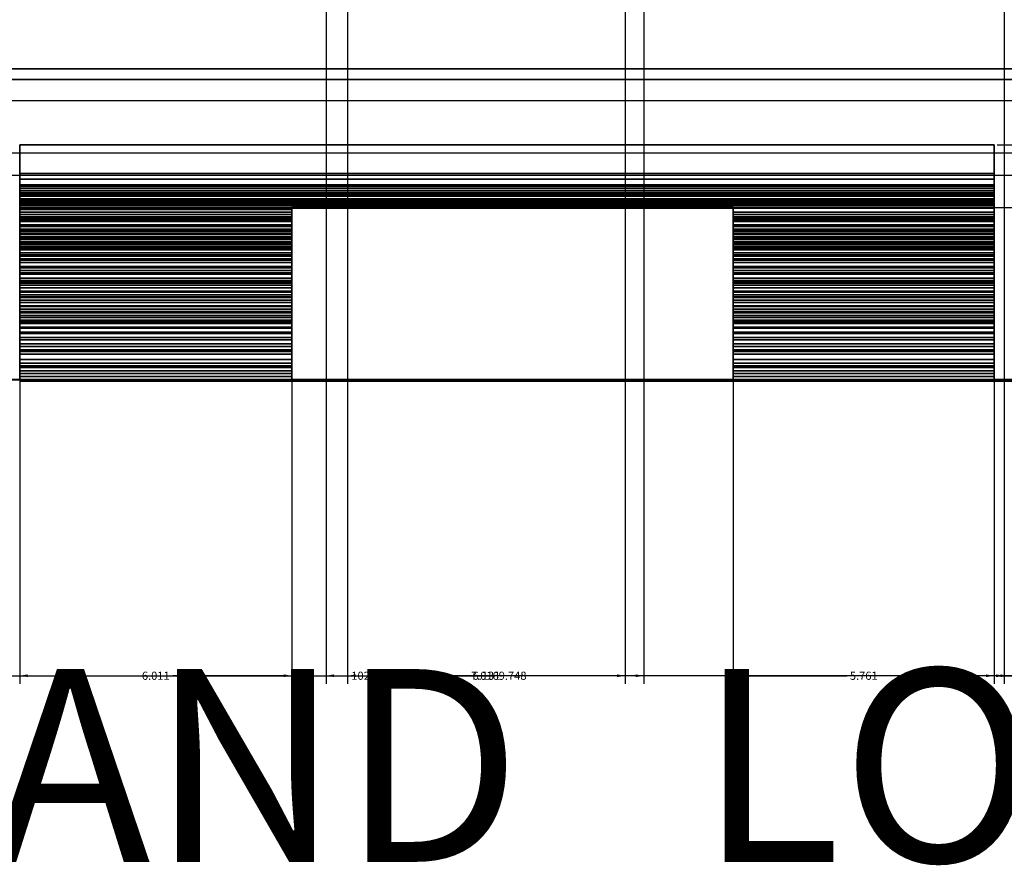
# Model space of a CAD drawing. Units: inches. Extents: x -10 to 130, y -32 to 34.
# Tile 12 of 22: x 49.15 to 70.9, y -32.13 to -13.47. Entities that reach past the tile are written whole.
import ezdxf

# ---------------------------------------------------------------- set-up
doc = ezdxf.new("R2010")
doc.units = ezdxf.units.IN
doc.header["$MEASUREMENT"] = 0
for name, color, linetype, lineweight in [('A-ANNO-DIMS', 2, 'Continuous', 18), ('A-ANNO-TEXT', 7, 'Continuous', 25), ('A-ELEV', 7, 'Continuous', 35)]:
    doc.layers.add(name, color=color, linetype=linetype, lineweight=lineweight)
doc.styles.get("Standard").update_dxf_attribs({"font": 'arial.ttf'})
doc.dimstyles.get("Standard").update_dxf_attribs({"dimtxt": 0.18, "dimasz": 0.18, "dimexe": 0.18, "dimexo": 0.0625, "dimgap": 0.09, "dimtad": 0, "dimtih": 1, "dimtoh": 1, "dimdec": 4, "dimzin": 0, "dimdsep": 46, "dimtxsty": 'Standard', "dimcen": 0.09, "dimadec": 0, "dimazin": 0, "dimtfac": 1, "dimtdec": 4, "dimtofl": 0, "dimtmove": 0, "dimatfit": 3, "dimfxl": 1, "dimtolj": 1, "dimtzin": 0, "dimarcsym": 0})

# ---------------------------------------------------------------- blocks, each defined once
blk = doc.blocks.new('*D1')
at = {"layer": 'A-ANNO-DIMS', "color": 0, "lineweight": -2, "transparency": 16777216}
for p, q in [((5.634, -13.647), (5.634, -28.129)), ((107.933, -21.477), (107.933, -28.129)), ((5.814, -27.949), (56.398, -27.949)), ((107.753, -27.949), (57.169, -27.949))]:
    blk.add_line(p, q, dxfattribs=at)
at = {"layer": 'A-ANNO-DIMS', "color": 0, "transparency": 16777216}
for points in [[(5.814, -27.919), (5.814, -27.979), (5.634, -27.949)], [(107.753, -27.919), (107.753, -27.979), (107.933, -27.949)]]:
    blk.add_solid(points, dxfattribs=at)
at = {"layer": 'Defpoints', "color": 0, "transparency": 16777216}
for p in [(5.634, -13.584), (107.933, -21.414), (107.933, -27.949)]:
    blk.add_point(p, dxfattribs=at)
at = {"layer": 'A-ANNO-DIMS', "color": 0, "transparency": 16777216, "insert": (56.784, -27.949), "char_height": 0.18, "attachment_point": 5}
blk.add_mtext('\\A1;102.3', dxfattribs=at)
blk = doc.blocks.new('*D2')
at = {"layer": 'A-ANNO-DIMS', "color": 0, "lineweight": -2, "transparency": 16777216}
for p, q in [((68.738, 27.199), (129.508, 27.199)), ((129.328, 27.019), (129.328, 3.074)), ((129.328, -21.234), (129.328, 2.71)), ((107.996, -21.414), (129.508, -21.414))]:
    blk.add_line(p, q, dxfattribs=at)
at = {"layer": 'A-ANNO-DIMS', "color": 0, "transparency": 16777216}
for points in [[(129.298, 27.019), (129.358, 27.019), (129.328, 27.199)], [(129.298, -21.234), (129.358, -21.234), (129.328, -21.414)]]:
    blk.add_solid(points, dxfattribs=at)
at = {"layer": 'Defpoints', "color": 0, "transparency": 16777216}
for p in [(68.676, 27.199), (129.328, 27.199), (107.933, -21.414)]:
    blk.add_point(p, dxfattribs=at)
at = {"layer": 'A-ANNO-DIMS', "color": 0, "transparency": 16777216, "insert": (129.328, 2.892), "char_height": 0.18, "attachment_point": 5}
blk.add_mtext('\\A1;48.61', dxfattribs=at)
blk = doc.blocks.new('*D47')
at = {"layer": 'A-ANNO-DIMS', "color": 0, "lineweight": -2, "transparency": 16777216}
for p, q in [((35.567, -12.534), (129.508, -12.534)), ((129.328, -12.714), (129.328, -16.792)), ((129.328, -21.234), (129.328, -17.156)), ((32.034, -21.414), (129.508, -21.414))]:
    blk.add_line(p, q, dxfattribs=at)
at = {"layer": 'A-ANNO-DIMS', "color": 0, "transparency": 16777216}
for points in [[(129.298, -12.714), (129.358, -12.714), (129.328, -12.534)], [(129.298, -21.234), (129.358, -21.234), (129.328, -21.414)]]:
    blk.add_solid(points, dxfattribs=at)
at = {"layer": 'Defpoints', "color": 0, "transparency": 16777216}
for p in [(35.505, -12.534), (31.971, -21.414), (129.328, -21.414)]:
    blk.add_point(p, dxfattribs=at)
at = {"layer": 'A-ANNO-DIMS', "color": 0, "transparency": 16777216, "insert": (129.328, -16.974), "char_height": 0.18, "attachment_point": 5}
blk.add_mtext('\\A1;8.88', dxfattribs=at)
blk = doc.blocks.new('*D52')
at = {"layer": 'A-ANNO-DIMS', "color": 0, "lineweight": -2, "transparency": 16777216}
for p, q in [((49.153, -16.297), (49.153, -28.129)), ((55.165, -17.677), (55.165, -28.129)), ((49.333, -27.949), (51.782, -27.949)), ((54.985, -27.949), (52.536, -27.949))]:
    blk.add_line(p, q, dxfattribs=at)
at = {"layer": 'A-ANNO-DIMS', "color": 0, "transparency": 16777216}
for points in [[(49.333, -27.919), (49.333, -27.979), (49.153, -27.949)], [(54.985, -27.919), (54.985, -27.979), (55.165, -27.949)]]:
    blk.add_solid(points, dxfattribs=at)
at = {"layer": 'Defpoints', "color": 0, "transparency": 16777216}
for p in [(49.153, -16.234), (55.165, -17.615), (55.165, -27.949)]:
    blk.add_point(p, dxfattribs=at)
at = {"layer": 'A-ANNO-DIMS', "color": 0, "transparency": 16777216, "insert": (52.159, -27.949), "char_height": 0.18, "attachment_point": 5}
blk.add_mtext('\\A1;6.011', dxfattribs=at)
blk = doc.blocks.new('*D53')
at = {"layer": 'A-ANNO-DIMS', "color": 0, "lineweight": -2, "transparency": 16777216}
for p, q in [((55.165, -17.677), (55.165, -28.129)), ((64.913, -17.677), (64.913, -28.129)), ((55.345, -27.949), (59.645, -27.949)), ((64.733, -27.949), (60.433, -27.949))]:
    blk.add_line(p, q, dxfattribs=at)
at = {"layer": 'A-ANNO-DIMS', "color": 0, "transparency": 16777216}
for points in [[(55.345, -27.919), (55.345, -27.979), (55.165, -27.949)], [(64.733, -27.919), (64.733, -27.979), (64.913, -27.949)]]:
    blk.add_solid(points, dxfattribs=at)
at = {"layer": 'Defpoints', "color": 0, "transparency": 16777216}
for p in [(55.165, -17.615), (64.913, -17.615), (64.913, -27.949)]:
    blk.add_point(p, dxfattribs=at)
at = {"layer": 'A-ANNO-DIMS', "color": 0, "transparency": 16777216, "insert": (60.039, -27.949), "char_height": 0.18, "attachment_point": 5}
blk.add_mtext('\\A1;9.748', dxfattribs=at)
blk = doc.blocks.new('*D54')
at = {"layer": 'A-ANNO-DIMS', "color": 0, "lineweight": -2, "transparency": 16777216}
for p, q in [((70.674, -16.297), (70.674, -28.129)), ((64.913, -17.677), (64.913, -28.129)), ((65.093, -27.949), (67.417, -27.949)), ((70.494, -27.949), (68.17, -27.949))]:
    blk.add_line(p, q, dxfattribs=at)
at = {"layer": 'A-ANNO-DIMS', "color": 0, "transparency": 16777216}
for points in [[(65.093, -27.919), (65.093, -27.979), (64.913, -27.949)], [(70.494, -27.919), (70.494, -27.979), (70.674, -27.949)]]:
    blk.add_solid(points, dxfattribs=at)
at = {"layer": 'Defpoints', "color": 0, "transparency": 16777216}
for p in [(70.674, -16.234), (64.913, -17.615), (70.674, -27.949)]:
    blk.add_point(p, dxfattribs=at)
at = {"layer": 'A-ANNO-DIMS', "color": 0, "transparency": 16777216, "insert": (67.794, -27.949), "char_height": 0.18, "attachment_point": 5}
blk.add_mtext('\\A1;5.761', dxfattribs=at)
blk = doc.blocks.new('*D55')
at = {"layer": 'A-ANNO-DIMS', "color": 0, "lineweight": -2, "transparency": 16777216}
for p, q in [((72.406, -14.617), (72.406, -28.129)), ((70.674, -16.297), (70.674, -28.129)), ((70.854, -27.949), (71.156, -27.949)), ((72.226, -27.949), (71.925, -27.949))]:
    blk.add_line(p, q, dxfattribs=at)
at = {"layer": 'A-ANNO-DIMS', "color": 0, "transparency": 16777216}
for points in [[(70.854, -27.919), (70.854, -27.979), (70.674, -27.949)], [(72.226, -27.919), (72.226, -27.979), (72.406, -27.949)]]:
    blk.add_solid(points, dxfattribs=at)
at = {"layer": 'Defpoints', "color": 0, "transparency": 16777216}
for p in [(72.406, -14.555), (70.674, -16.234), (72.406, -27.949)]:
    blk.add_point(p, dxfattribs=at)
at = {"layer": 'A-ANNO-DIMS', "color": 0, "transparency": 16777216, "insert": (71.54, -27.949), "char_height": 0.18, "attachment_point": 5}
blk.add_mtext('\\A1;1.732', dxfattribs=at)
blk = doc.blocks.new('*D58')
at = {"layer": 'A-ANNO-DIMS', "color": 0, "lineweight": -2, "transparency": 16777216}
for p, q in [((70.737, -16.234), (129.508, -16.234)), ((129.328, -16.414), (129.328, -18.66)), ((129.328, -21.269), (129.328, -19.024)), ((70.737, -21.449), (129.508, -21.449))]:
    blk.add_line(p, q, dxfattribs=at)
at = {"layer": 'A-ANNO-DIMS', "color": 0, "transparency": 16777216}
for points in [[(129.298, -16.414), (129.358, -16.414), (129.328, -16.234)], [(129.298, -21.269), (129.358, -21.269), (129.328, -21.449)]]:
    blk.add_solid(points, dxfattribs=at)
at = {"layer": 'Defpoints', "color": 0, "transparency": 16777216}
for p in [(70.674, -16.234), (70.674, -21.449), (129.328, -21.449)]:
    blk.add_point(p, dxfattribs=at)
at = {"layer": 'A-ANNO-DIMS', "color": 0, "transparency": 16777216, "insert": (129.328, -18.842), "char_height": 0.18, "attachment_point": 5}
blk.add_mtext('\\A1;5.215', dxfattribs=at)
blk = doc.blocks.new('*D59')
at = {"layer": 'A-ANNO-DIMS', "color": 0, "lineweight": -2, "transparency": 16777216}
for p, q in [((64.975, -17.615), (129.508, -17.615)), ((129.328, -17.795), (129.328, -19.35)), ((129.328, -21.269), (129.328, -19.714)), ((64.975, -21.449), (129.508, -21.449))]:
    blk.add_line(p, q, dxfattribs=at)
at = {"layer": 'A-ANNO-DIMS', "color": 0, "transparency": 16777216}
for points in [[(129.298, -17.795), (129.358, -17.795), (129.328, -17.615)], [(129.298, -21.269), (129.358, -21.269), (129.328, -21.449)]]:
    blk.add_solid(points, dxfattribs=at)
at = {"layer": 'Defpoints', "color": 0, "transparency": 16777216}
for p in [(64.913, -17.615), (64.913, -21.449), (129.328, -21.449)]:
    blk.add_point(p, dxfattribs=at)
at = {"layer": 'A-ANNO-DIMS', "color": 0, "transparency": 16777216, "insert": (129.328, -19.532), "char_height": 0.18, "attachment_point": 5}
blk.add_mtext('\\A1;3.835', dxfattribs=at)
blk = doc.blocks.new('*D64')
at = {"layer": 'A-ANNO-DIMS', "color": 0, "lineweight": -2, "transparency": 16777216}
for p, q in [((82.315, -15.264), (-9.564, -15.264)), ((-9.384, -15.444), (-9.384, -15.659)), ((-9.384, -16.237), (-9.384, -16.022)), ((82.315, -16.417), (-9.564, -16.417))]:
    blk.add_line(p, q, dxfattribs=at)
at = {"layer": 'A-ANNO-DIMS', "color": 0, "transparency": 16777216}
for points in [[(-9.414, -15.444), (-9.354, -15.444), (-9.384, -15.264)], [(-9.414, -16.237), (-9.354, -16.237), (-9.384, -16.417)]]:
    blk.add_solid(points, dxfattribs=at)
at = {"layer": 'Defpoints', "color": 0, "transparency": 16777216}
for p in [(82.377, -15.264), (-9.384, -16.417), (82.377, -16.417)]:
    blk.add_point(p, dxfattribs=at)
at = {"layer": 'A-ANNO-DIMS', "color": 0, "transparency": 16777216, "insert": (-9.384, -15.841), "char_height": 0.18, "attachment_point": 5}
blk.add_mtext('\\A1;1.15', dxfattribs=at)
blk = doc.blocks.new('*D65')
at = {"layer": 'A-ANNO-DIMS', "color": 0, "lineweight": -2, "transparency": 16777216}
for p, q in [((82.315, -16.417), (-9.564, -16.417)), ((-9.384, -16.597), (-9.384, -18.734)), ((-9.384, -21.234), (-9.384, -19.097)), ((80.669, -21.414), (-9.564, -21.414))]:
    blk.add_line(p, q, dxfattribs=at)
at = {"layer": 'A-ANNO-DIMS', "color": 0, "transparency": 16777216}
for points in [[(-9.414, -16.597), (-9.354, -16.597), (-9.384, -16.417)], [(-9.414, -21.234), (-9.354, -21.234), (-9.384, -21.414)]]:
    blk.add_solid(points, dxfattribs=at)
at = {"layer": 'Defpoints', "color": 0, "transparency": 16777216}
for p in [(-9.384, -16.417), (82.377, -16.417), (80.731, -21.414)]:
    blk.add_point(p, dxfattribs=at)
at = {"layer": 'A-ANNO-DIMS', "color": 0, "transparency": 16777216, "insert": (-9.384, -18.916), "char_height": 0.18, "attachment_point": 5}
blk.add_mtext('\\A1;4.998', dxfattribs=at)
blk = doc.blocks.new('*D69')
at = {"layer": 'A-ANNO-DIMS', "color": 0, "lineweight": -2, "transparency": 16777216}
for p, q in [((89.095, -16.906), (-9.564, -16.906)), ((-9.384, -17.086), (-9.384, -18.979)), ((-9.384, -21.234), (-9.384, -19.342)), ((89.095, -21.414), (-9.564, -21.414))]:
    blk.add_line(p, q, dxfattribs=at)
at = {"layer": 'A-ANNO-DIMS', "color": 0, "transparency": 16777216}
for points in [[(-9.414, -17.086), (-9.354, -17.086), (-9.384, -16.906)], [(-9.414, -21.234), (-9.354, -21.234), (-9.384, -21.414)]]:
    blk.add_solid(points, dxfattribs=at)
at = {"layer": 'Defpoints', "color": 0, "transparency": 16777216}
for p in [(89.158, -16.906), (-9.384, -21.414), (89.158, -21.414)]:
    blk.add_point(p, dxfattribs=at)
at = {"layer": 'A-ANNO-DIMS', "color": 0, "transparency": 16777216, "insert": (-9.384, -19.16), "char_height": 0.18, "attachment_point": 5}
blk.add_mtext('\\A1;4.508', dxfattribs=at)
blk = doc.blocks.new('*D72')
at = {"layer": 'A-ANNO-DIMS', "color": 0, "lineweight": -2, "transparency": 16777216}
for p, q in [((55.918, 16.529), (55.918, -28.129)), ((62.934, 16.482), (62.934, -28.129)), ((56.098, -27.949), (59.033, -27.949)), ((62.754, -27.949), (59.819, -27.949))]:
    blk.add_line(p, q, dxfattribs=at)
at = {"layer": 'A-ANNO-DIMS', "color": 0, "transparency": 16777216}
for points in [[(56.098, -27.919), (56.098, -27.979), (55.918, -27.949)], [(62.754, -27.919), (62.754, -27.979), (62.934, -27.949)]]:
    blk.add_solid(points, dxfattribs=at)
at = {"layer": 'Defpoints', "color": 0, "transparency": 16777216}
for p in [(55.918, 16.591), (62.934, 16.545), (62.934, -27.949)]:
    blk.add_point(p, dxfattribs=at)
at = {"layer": 'A-ANNO-DIMS', "color": 0, "transparency": 16777216, "insert": (59.426, -27.949), "char_height": 0.18, "attachment_point": 5}
blk.add_mtext('\\A1;7.016', dxfattribs=at)
blk = doc.blocks.new('*D73')
at = {"layer": 'A-ANNO-DIMS', "color": 0, "lineweight": -2, "transparency": 16777216}
for p, q in [((56.395, 16.255), (56.395, -28.129)), ((62.526, 16.255), (62.526, -28.129)), ((56.575, -27.949), (59.083, -27.949)), ((62.346, -27.949), (59.837, -27.949))]:
    blk.add_line(p, q, dxfattribs=at)
at = {"layer": 'A-ANNO-DIMS', "color": 0, "transparency": 16777216}
for points in [[(56.575, -27.919), (56.575, -27.979), (56.395, -27.949)], [(62.346, -27.919), (62.346, -27.979), (62.526, -27.949)]]:
    blk.add_solid(points, dxfattribs=at)
at = {"layer": 'Defpoints', "color": 0, "transparency": 16777216}
for p in [(56.395, 16.317), (62.526, 16.317), (62.526, -27.949)]:
    blk.add_point(p, dxfattribs=at)
at = {"layer": 'A-ANNO-DIMS', "color": 0, "transparency": 16777216, "insert": (59.46, -27.949), "char_height": 0.18, "attachment_point": 5}
blk.add_mtext('\\A1;6.131', dxfattribs=at)
blk = doc.blocks.new('*D155')
at = {"layer": 'A-ANNO-DIMS', "color": 0, "lineweight": -2, "transparency": 16777216}
for p, q in [((70.897993, 1.448166), (70.897993, -28.129305)), ((71.936707, 1.448166), (71.936707, -28.129305)), ((70.717993, -27.949305), (70.537993, -27.949305)), ((72.116707, -27.949305), (72.296707, -27.949305))]:
    blk.add_line(p, q, dxfattribs=at)
at = {"layer": 'A-ANNO-DIMS', "color": 0, "transparency": 16777216}
for points in [[(70.717993, -27.919305), (70.717993, -27.979305), (70.897993, -27.949305)], [(72.116707, -27.919305), (72.116707, -27.979305), (71.936707, -27.949305)]]:
    blk.add_solid(points, dxfattribs=at)
at = {"layer": 'Defpoints', "color": 0, "transparency": 16777216}
for p in [(70.897993, 1.510666), (71.936707, 1.510666), (71.936707, -27.949305)]:
    blk.add_point(p, dxfattribs=at)
at = {"layer": 'A-ANNO-DIMS', "color": 0, "transparency": 16777216, "insert": (71.41735, -27.949305), "char_height": 0.18, "attachment_point": 5}
blk.add_mtext('\\A1;1.039', dxfattribs=at)

msp = doc.modelspace()

# ---------------------------------------------------------------- linework, layer by layer
at = {"layer": 'A-ELEV'}
for p, q in [((54.1471, -14.555), (47.3492, -14.555)), ((54.1471, -14.555), (64.8443, -14.555)), ((64.8443, -14.555), (72.4063, -14.555)), ((54.1471, -14.7925), (47.3492, -14.7925)), ((54.1471, -14.7925), (64.8443, -14.7925)), ((64.8443, -14.7925), (72.4063, -14.7925)), ((49.1533, -16.2341), (70.6743, -16.2341)), ((49.1533, -16.2341), (49.1533, -21.4145)), ((70.6743, -16.2341), (70.6743, -21.4145)), ((49.1533, -16.867), (70.6743, -16.867)), ((49.1533, -16.987), (70.6743, -16.987)), ((49.1533, -17.1115), (70.6743, -17.1115)), ((49.1533, -17.1249), (70.6743, -17.1249)), ((49.1533, -17.1447), (70.6743, -17.1447)), ((49.1533, -17.1843), (70.6743, -17.1843)), ((49.1533, -17.236), (70.6743, -17.236)), ((49.1533, -17.2835), (70.6743, -17.2835)), ((49.1533, -17.3231), (70.6743, -17.3231)), ((49.1533, -17.3427), (70.6743, -17.3427)), ((49.1533, -17.3429), (70.6743, -17.3429)), ((49.1533, -17.3628), (70.6743, -17.3628)), ((49.1533, -17.4222), (70.6743, -17.4222)), ((49.1533, -17.442), (70.6743, -17.442)), ((49.1533, -17.4494), (70.6743, -17.4494)), ((49.1533, -17.4817), (70.6743, -17.4817)), ((49.1533, -17.5213), (70.6743, -17.5213)), ((49.1533, -17.5383), (70.6743, -17.5383)), ((49.1533, -17.5517), (70.6743, -17.5517)), ((49.1533, -17.561), (70.6743, -17.561)), ((49.1533, -17.5808), (70.6743, -17.5808)), ((49.1533, -17.6205), (70.6743, -17.6205)), ((49.1533, -17.6272), (70.6743, -17.6272)), ((49.1533, -17.6601), (55.1648, -17.6601)), ((49.1533, -17.7196), (55.1648, -17.7196)), ((49.1533, -17.7196), (55.1648, -17.7196)), ((49.1533, -17.7695), (55.1648, -17.7695)), ((49.1533, -17.8187), (55.1648, -17.8187)), ((55.1648, -21.4493), (55.1648, -17.6146)), ((55.1648, -17.6146), (64.913, -17.6146)), ((64.913, -17.6146), (64.913, -21.4493)), ((64.913, -17.7196), (70.6743, -17.7196)), ((64.913, -17.7196), (70.6743, -17.7196)), ((64.913, -17.7695), (70.6743, -17.7695)), ((64.913, -17.8187), (70.6743, -17.8187)), ((49.1533, -17.8385), (55.1648, -17.8385)), ((49.1533, -17.8584), (55.1648, -17.8584)), ((49.1533, -17.8584), (55.1648, -17.8584)), ((49.1533, -17.8931), (55.1648, -17.8931)), ((49.1533, -17.9178), (55.1648, -17.9178)), ((49.1533, -17.9215), (55.1648, -17.9215)), ((49.1533, -17.9971), (55.1648, -17.9971)), ((49.1533, -18.0069), (55.1648, -18.0069)), ((49.1533, -18.017), (55.1648, -18.017)), ((49.1533, -18.0353), (55.1648, -18.0353)), ((49.1533, -18.0353), (55.1648, -18.0353)), ((64.913, -17.8385), (70.6743, -17.8385)), ((64.913, -17.8584), (70.6743, -17.8584)), ((64.913, -17.8584), (70.6743, -17.8584)), ((64.913, -17.8931), (70.6743, -17.8931)), ((64.913, -17.9178), (70.6743, -17.9178)), ((64.913, -17.9215), (70.6743, -17.9215)), ((64.913, -17.9971), (70.6743, -17.9971)), ((64.913, -18.0069), (70.6743, -18.0069)), ((64.913, -18.017), (70.6743, -18.017)), ((64.913, -18.0353), (70.6743, -18.0353)), ((64.913, -18.0353), (70.6743, -18.0353)), ((49.1533, -18.0963), (55.1648, -18.0963)), ((49.1533, -18.1161), (55.1648, -18.1161)), ((49.1533, -18.1359), (55.1648, -18.1359)), ((49.1533, -18.1491), (55.1648, -18.1491)), ((49.1533, -18.1491), (55.1648, -18.1491)), ((49.1533, -18.1954), (55.1648, -18.1954)), ((49.1533, -18.1954), (55.1648, -18.1954)), ((49.1533, -18.206), (55.1648, -18.206)), ((49.1533, -18.206), (55.1648, -18.206)), ((49.1533, -18.2549), (55.1648, -18.2549)), ((64.913, -18.0963), (70.6743, -18.0963)), ((64.913, -18.1161), (70.6743, -18.1161)), ((64.913, -18.1359), (70.6743, -18.1359)), ((64.913, -18.1491), (70.6743, -18.1491)), ((64.913, -18.1491), (70.6743, -18.1491)), ((64.913, -18.1954), (70.6743, -18.1954)), ((64.913, -18.1954), (70.6743, -18.1954)), ((64.913, -18.206), (70.6743, -18.206)), ((64.913, -18.206), (70.6743, -18.206)), ((64.913, -18.2549), (70.6743, -18.2549)), ((49.1533, -18.2914), (55.1648, -18.2914)), ((49.1533, -18.3143), (55.1648, -18.3143)), ((49.1533, -18.3198), (55.1648, -18.3198)), ((49.1533, -18.3198), (55.1648, -18.3198)), ((49.1533, -18.3207), (55.1648, -18.3207)), ((49.1533, -18.3738), (55.1648, -18.3738)), ((49.1533, -18.3936), (55.1648, -18.3936)), ((49.1533, -18.4052), (55.1648, -18.4052)), ((49.1533, -18.4052), (55.1648, -18.4052)), ((49.1533, -18.4333), (55.1648, -18.4333)), ((49.1533, -18.4729), (55.1648, -18.4729)), ((49.1533, -18.4729), (55.1648, -18.4729)), ((64.913, -18.2914), (70.6743, -18.2914)), ((64.913, -18.3143), (70.6743, -18.3143)), ((64.913, -18.3198), (70.6743, -18.3198)), ((64.913, -18.3198), (70.6743, -18.3198)), ((64.913, -18.3207), (70.6743, -18.3207)), ((64.913, -18.3738), (70.6743, -18.3738)), ((64.913, -18.3936), (70.6743, -18.3936)), ((64.913, -18.4052), (70.6743, -18.4052)), ((64.913, -18.4052), (70.6743, -18.4052)), ((64.913, -18.4333), (70.6743, -18.4333)), ((64.913, -18.4729), (70.6743, -18.4729)), ((64.913, -18.4729), (70.6743, -18.4729)), ((49.1533, -18.4986), (55.1648, -18.4986)), ((49.1533, -18.519), (55.1648, -18.519)), ((49.1533, -18.519), (55.1648, -18.519)), ((49.1533, -18.519), (55.1648, -18.519)), ((49.1533, -18.519), (55.1648, -18.519)), ((49.1533, -18.5474), (55.1648, -18.5474)), ((49.1533, -18.5522), (55.1648, -18.5522)), ((49.1533, -18.6117), (55.1648, -18.6117)), ((49.1533, -18.6612), (55.1648, -18.6612)), ((49.1533, -18.6897), (55.1648, -18.6897)), ((49.1533, -18.691), (55.1648, -18.691)), ((64.913, -18.4986), (70.6743, -18.4986)), ((64.913, -18.519), (70.6743, -18.519)), ((64.913, -18.519), (70.6743, -18.519)), ((64.913, -18.519), (70.6743, -18.519)), ((64.913, -18.519), (70.6743, -18.519)), ((64.913, -18.5474), (70.6743, -18.5474)), ((64.913, -18.5522), (70.6743, -18.5522)), ((64.913, -18.6117), (70.6743, -18.6117)), ((64.913, -18.6612), (70.6743, -18.6612)), ((64.913, -18.6897), (70.6743, -18.6897)), ((64.913, -18.691), (70.6743, -18.691)), ((49.1533, -18.7466), (55.1648, -18.7466)), ((49.1533, -18.7505), (55.1648, -18.7505)), ((49.1533, -18.775), (55.1648, -18.775)), ((49.1533, -18.775), (55.1648, -18.775)), ((49.1533, -18.8298), (55.1648, -18.8298)), ((49.1533, -18.9173), (55.1648, -18.9173)), ((64.913, -18.7466), (70.6743, -18.7466)), ((64.913, -18.7505), (70.6743, -18.7505)), ((64.913, -18.775), (70.6743, -18.775)), ((64.913, -18.775), (70.6743, -18.775)), ((64.913, -18.8298), (70.6743, -18.8298)), ((64.913, -18.9173), (70.6743, -18.9173)), ((49.1533, -18.9289), (55.1648, -18.9289)), ((49.1533, -18.9457), (55.1648, -18.9457)), ((49.1533, -19.0026), (55.1648, -19.0026)), ((49.1533, -19.0595), (55.1648, -19.0595)), ((49.1533, -19.088), (55.1648, -19.088)), ((64.913, -18.9289), (70.6743, -18.9289)), ((64.913, -18.9457), (70.6743, -18.9457)), ((64.913, -19.0026), (70.6743, -19.0026)), ((64.913, -19.0595), (70.6743, -19.0595)), ((64.913, -19.088), (70.6743, -19.088)), ((49.1533, -19.1733), (55.1648, -19.1733)), ((49.1533, -19.2263), (55.1648, -19.2263)), ((49.1533, -19.2461), (55.1648, -19.2461)), ((49.1533, -19.2871), (55.1648, -19.2871)), ((49.1533, -19.2871), (55.1648, -19.2871)), ((49.1533, -19.3254), (55.1648, -19.3254)), ((64.913, -19.1733), (70.6743, -19.1733)), ((64.913, -19.2263), (70.6743, -19.2263)), ((64.913, -19.2461), (70.6743, -19.2461)), ((64.913, -19.2871), (70.6743, -19.2871)), ((64.913, -19.2871), (70.6743, -19.2871)), ((64.913, -19.3254), (70.6743, -19.3254)), ((49.1533, -19.3848), (55.1648, -19.3848)), ((49.1533, -19.4578), (55.1648, -19.4578)), ((49.1533, -19.4863), (55.1648, -19.4863)), ((49.1533, -19.5434), (55.1648, -19.5434)), ((64.913, -19.3848), (70.6743, -19.3848)), ((64.913, -19.4578), (70.6743, -19.4578)), ((64.913, -19.4863), (70.6743, -19.4863)), ((64.913, -19.5434), (70.6743, -19.5434)), ((49.1533, -19.5831), (55.1648, -19.5831)), ((49.1533, -19.6001), (55.1648, -19.6001)), ((49.1533, -19.657), (55.1648, -19.657)), ((49.1533, -19.7139), (55.1648, -19.7139)), ((49.1533, -19.7813), (55.1648, -19.7813)), ((64.913, -19.5831), (70.6743, -19.5831)), ((64.913, -19.6001), (70.6743, -19.6001)), ((64.913, -19.657), (70.6743, -19.657)), ((64.913, -19.7139), (70.6743, -19.7139)), ((64.913, -19.7813), (70.6743, -19.7813)), ((49.1533, -19.8012), (55.1648, -19.8012)), ((49.1533, -19.8606), (55.1648, -19.8606)), ((49.1533, -19.913), (55.1648, -19.913)), ((49.1533, -19.9399), (55.1648, -19.9399)), ((49.1533, -19.9415), (55.1648, -19.9415)), ((49.1533, -19.9984), (55.1648, -19.9984)), ((64.913, -19.8012), (70.6743, -19.8012)), ((64.913, -19.8606), (70.6743, -19.8606)), ((64.913, -19.913), (70.6743, -19.913)), ((64.913, -19.9399), (70.6743, -19.9399)), ((64.913, -19.9415), (70.6743, -19.9415)), ((64.913, -19.9984), (70.6743, -19.9984)), ((49.1533, -20.0391), (55.1648, -20.0391)), ((49.1533, -20.0985), (55.1648, -20.0985)), ((49.1533, -20.1406), (55.1648, -20.1406)), ((49.1533, -20.158), (55.1648, -20.158)), ((49.1533, -20.1778), (55.1648, -20.1778)), ((64.913, -20.0391), (70.6743, -20.0391)), ((64.913, -20.0985), (70.6743, -20.0985)), ((64.913, -20.1406), (70.6743, -20.1406)), ((64.913, -20.158), (70.6743, -20.158)), ((64.913, -20.1778), (70.6743, -20.1778)), ((49.1533, -20.2544), (55.1648, -20.2544)), ((49.1533, -20.2544), (55.1648, -20.2544)), ((49.1533, -20.2769), (55.1648, -20.2769)), ((49.1533, -20.3682), (55.1648, -20.3682)), ((49.1533, -20.3967), (55.1648, -20.3967)), ((64.913, -20.2544), (70.6743, -20.2544)), ((64.913, -20.2544), (70.6743, -20.2544)), ((64.913, -20.2769), (70.6743, -20.2769)), ((64.913, -20.3682), (70.6743, -20.3682)), ((64.913, -20.3967), (70.6743, -20.3967)), ((49.1533, -20.482), (55.1648, -20.482)), ((49.1533, -20.5389), (55.1648, -20.5389)), ((49.1533, -20.6243), (55.1648, -20.6243)), ((64.913, -20.482), (70.6743, -20.482)), ((64.913, -20.5389), (70.6743, -20.5389)), ((64.913, -20.6243), (70.6743, -20.6243)), ((49.1533, -20.6812), (55.1648, -20.6812)), ((49.1533, -20.7527), (55.1648, -20.7527)), ((49.1533, -20.795), (55.1648, -20.795)), ((49.1533, -20.795), (55.1648, -20.795)), ((49.1533, -20.8519), (55.1648, -20.8519)), ((49.1533, -20.8519), (55.1648, -20.8519)), ((64.913, -20.6812), (70.6743, -20.6812)), ((64.913, -20.7527), (70.6743, -20.7527)), ((64.913, -20.795), (70.6743, -20.795)), ((64.913, -20.795), (70.6743, -20.795)), ((64.913, -20.8519), (70.2773, -20.8519)), ((64.913, -20.8519), (70.6743, -20.8519)), ((49.1533, -20.9657), (55.1648, -20.9657)), ((49.1533, -21.051), (55.1648, -21.051)), ((64.913, -20.9657), (70.6743, -20.9657)), ((64.913, -21.051), (70.6743, -21.051)), ((49.1533, -21.1079), (55.1648, -21.1079)), ((49.1533, -21.1492), (55.1648, -21.1492)), ((49.1533, -21.2217), (55.1648, -21.2217)), ((49.1533, -21.2786), (55.1648, -21.2786)), ((49.1533, -21.2786), (55.1648, -21.2786)), ((64.913, -21.1079), (70.6743, -21.1079)), ((64.913, -21.1492), (70.6743, -21.1492)), ((64.913, -21.2217), (70.6743, -21.2217)), ((64.913, -21.2786), (70.6743, -21.2786)), ((64.913, -21.2786), (70.6743, -21.2786)), ((55.1648, -21.4145), (44.76, -21.4145)), ((49.1533, -21.3475), (55.1648, -21.3475)), ((49.1533, -21.4493), (55.1648, -21.4493)), ((55.1648, -21.4493), (64.913, -21.4493)), ((64.913, -21.3475), (70.6743, -21.3475)), ((74.492, -21.4145), (64.913, -21.4145)), ((64.913, -21.4493), (70.6743, -21.4493))]:
    msp.add_line(p, q, dxfattribs=at)

# ---------------------------------------------------------------- texts
at = {"layer": 'A-ANNO-TEXT'}
msp.add_text('REAR   ELEVATION    AND   LOGISTICS   HUB', height=4.256275, dxfattribs=at).set_placement((-5.4651, -32.0569))

# ---------------------------------------------------------------- dimensions: what is measured, and where the dimension line sits
at = {"layer": 'A-ANNO-DIMS'}
for base, p1, p2, override, picture, middle in [((129.3277, 27.1987), (107.9333, -21.4145), (68.6759, 27.1987), {"dimdec": 2, "dimlfac": 1, "dimrnd": 0, "dimzin": 0, "dimdsep": 46, "dimlunit": 2}, '*D2', (129.3277, 2.8921)), ((129.3277, -21.4145), (35.5046, -12.5339), (31.9712, -21.4145), {"dimdec": 2, "dimlfac": 1, "dimrnd": 0, "dimzin": 0, "dimdsep": 46, "dimlunit": 2}, '*D47', (129.3277, -16.9742)), ((-9.3836, -16.4166), (82.377, -15.2645), (82.377, -16.4166), {"dimdec": 2, "dimlfac": 1, "dimrnd": 0, "dimzin": 0, "dimdsep": 46, "dimlunit": 2}, '*D64', (-9.3836, -15.8406)), ((129.3277, -21.4493), (70.6743, -16.2341), (70.6743, -21.4493), {"dimdec": 3, "dimlfac": 1, "dimrnd": 0, "dimzin": 0, "dimdsep": 46, "dimlunit": 2}, '*D58', (129.3277, -18.8417)), ((-9.3836, -16.4166), (80.7314, -21.4145), (82.377, -16.4166), {"dimdec": 3, "dimlfac": 1, "dimrnd": 0, "dimzin": 0, "dimdsep": 46, "dimlunit": 2}, '*D65', (-9.3836, -18.9156)), ((-9.3836, -21.4145), (89.1578, -16.9063), (89.1578, -21.4145), {"dimdec": 3, "dimlfac": 1, "dimrnd": 0, "dimzin": 0, "dimdsep": 46, "dimlunit": 2}, '*D69', (-9.3836, -19.1604)), ((129.3277, -21.4493), (64.913, -17.6146), (64.913, -21.4493), {"dimdec": 3, "dimlfac": 1, "dimrnd": 0, "dimzin": 0, "dimdsep": 46, "dimlunit": 2}, '*D59', (129.3277, -19.532))]:
    dim = msp.add_linear_dim(base=base, p1=p1, p2=p2, angle=90, dimstyle='Standard', override=override, dxfattribs=at)
    dim.commit()
    dim.dimension.update_dxf_attribs({"geometry": picture, "text_midpoint": middle})
for base, p1, p2, override, picture, middle in [((62.9343, -27.9493), (55.9182, 16.5911), (62.9343, 16.5448), {"dimdec": 3, "dimlfac": 1, "dimrnd": 0, "dimzin": 0, "dimdsep": 46, "dimlunit": 2}, '*D72', (59.4263, -27.9493)), ((62.5256, -27.9493), (56.395, 16.3174), (62.5256, 16.3174), {"dimdec": 3, "dimlfac": 1, "dimrnd": 0, "dimzin": 0, "dimdsep": 46, "dimlunit": 2}, '*D73', (59.4603, -27.9493)), ((71.9367, -27.9493), (70.898, 1.5107), (71.9367, 1.5107), {"dimdec": 3, "dimlfac": 1, "dimrnd": 0, "dimzin": 0, "dimdsep": 46, "dimlunit": 2}, '*D155', (71.4173, -27.9493)), ((107.9333, -27.9493), (5.634, -13.5841), (107.9333, -21.4145), {"dimdec": 1, "dimlfac": 1, "dimrnd": 0, "dimzin": 0, "dimdsep": 46, "dimlunit": 2}, '*D1', (56.7837, -27.9493)), ((72.4063, -27.9493), (70.6743, -16.2341), (72.4063, -14.555), {"dimdec": 3, "dimlfac": 1, "dimrnd": 0, "dimzin": 0, "dimdsep": 46, "dimlunit": 2}, '*D55', (71.5403, -27.9493)), ((55.16483, -27.949305), (49.153331, -16.234138), (55.16483, -17.614631), {"dimdec": 3, "dimlfac": 1, "dimrnd": 0, "dimzin": 0, "dimdsep": 46, "dimlunit": 2}, '*D52', (52.159081, -27.949305)), ((70.6743, -27.9493), (64.913, -17.6146), (70.6743, -16.2341), {"dimdec": 3, "dimlfac": 1, "dimrnd": 0, "dimzin": 0, "dimdsep": 46, "dimlunit": 2}, '*D54', (67.7937, -27.9493)), ((64.913, -27.9493), (55.1648, -17.6146), (64.913, -17.6146), {"dimdec": 3, "dimlfac": 1, "dimrnd": 0, "dimzin": 0, "dimdsep": 46, "dimlunit": 2}, '*D53', (60.0389, -27.9493))]:
    dim = msp.add_linear_dim(base=base, p1=p1, p2=p2, dimstyle='Standard', override=override, dxfattribs=at)
    dim.commit()
    dim.dimension.update_dxf_attribs({"geometry": picture, "text_midpoint": middle})

doc.saveas('drawing.dxf')
